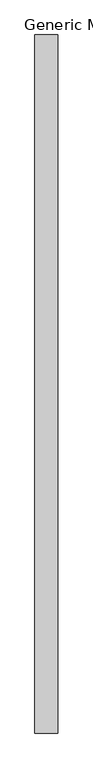
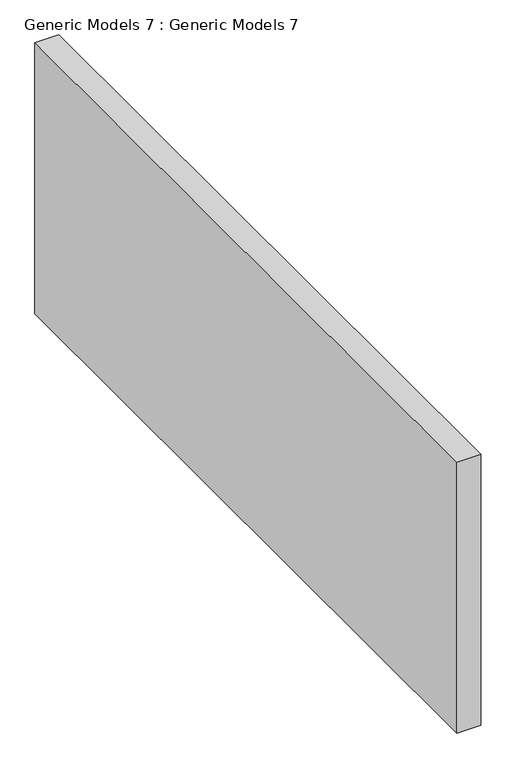
"""IFC4 building model written with IfcOpenShell, lengths in millimetres: proxy geometry, Generic Models 7 : Generic Models 7."""

from ifc_helpers import new_model, si_unit, frame, origin, place, context, project, spatial, polyline, outline, extrude, source, transform, mapped, element, save


def generic_models_7_generic_models_7_cfbcc48d(model_context):
    return source(origin(), model_context, "Body", "SweptSolid", [
        extrude(outline(polyline([(-6131.7781265, -4389.2142532), (-6131.7781265, -5944.8090355), (-6182.5781265, -5944.8090355), (-6182.5781265, -4389.2142532), (-6131.7781265, -4389.2142532)])), frame((0.0, 0.0, 5791.2), z_axis=(0.0, 0.0, 1.0), x_axis=(1.0, 0.0, 0.0)), (0.0, 0.0, 1.0), 609.6),
    ])


if __name__ == "__main__":
    model = new_model("IFC4")
    model_context = context("Model", 3, world=origin())
    ifc_project = project(units=[si_unit("LENGTHUNIT", "METRE", prefix="MILLI")], contexts=[model_context])
    site = spatial("IfcSite", under=ifc_project)
    building = spatial("IfcBuilding", under=site)
    placement = place(None, origin())
    generic_models_7_generic_models_7_shape = generic_models_7_generic_models_7_cfbcc48d(model_context)
    element("IfcBuildingElementProxy", 1, Name="Generic Models 7 : Generic Models 7", ObjectType="Generic Models 7 : Generic Models 7", at=placement, inside=building, context=model_context, shape_type="MappedRepresentation", body=[
        mapped(generic_models_7_generic_models_7_shape, transform((0.0, 0.0, 0.0), x_axis=(1.0, 0.0, 0.0), y_axis=(0.0, 1.0, 0.0), z_axis=(0.0, 0.0, 1.0))),
    ])
    save(model, "model.ifc")
